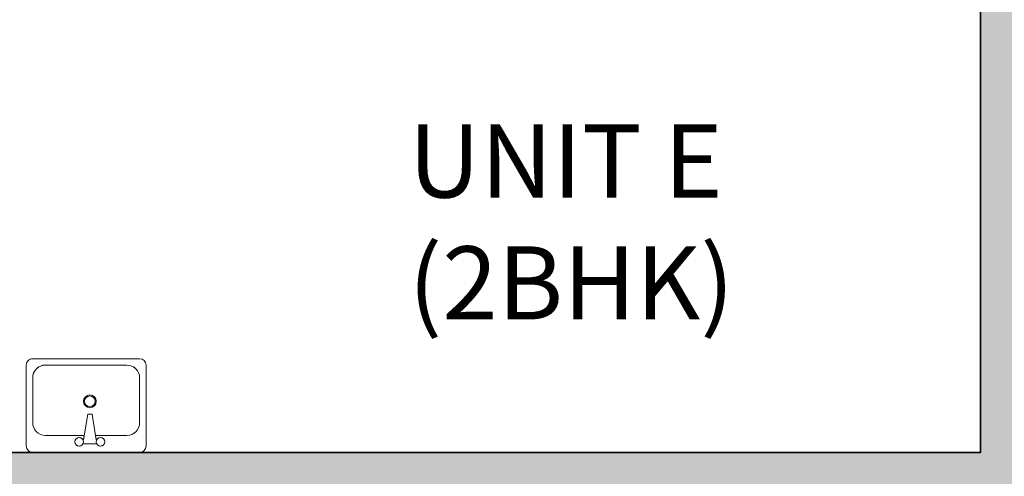
# Model space of a CAD drawing. Units: inches. Extents: x 2083 to 3317, y 1141 to 2115.
# Tile 102 of 256: x 2415 to 2600, y 1707 to 1794. Entities that reach past the tile are written whole.
import ezdxf

# ---------------------------------------------------------------- set-up
doc = ezdxf.new("R2010")
doc.units = ezdxf.units.IN
for name, color, linetype, lineweight in [('A-AREA-IDEN', 7, 'Continuous', 25), ('A-FLOR-FIXT', 9, 'Continuous', 18), ('A-WALL', 7, 'Continuous', 35)]:
    doc.layers.add(name, color=color, linetype=linetype, lineweight=lineweight)
doc.layers.add('A-WALL-PATT', color=251, linetype='Continuous', lineweight=13, true_color=0x636466)
doc.styles.add('DIM_FONT', font='TXT.shx', dxfattribs={"width": 0.8})
doc.styles.get("Standard").update_dxf_attribs({"font": 'arial.ttf'})

# ---------------------------------------------------------------- blocks, each defined once
blk = doc.blocks.new('A$C564A496C')
at = {"linetype": 'ByBlock'}
for p, q in [((543.2, 450), (30.7, 450)), ((0, 419.3), (0, 30.7)), ((238.5, 409.1), (299.8, 409.1)), ((238.5, 388.6), (258.9, 265.9)), ((279.4, 265.9), (299.8, 388.6)), ((573.8, 30.7), (573.8, 419.3)), ((92, 368.2), (243.6, 368.2)), ((294.7, 368.2), (481.8, 368.2)), ((30.7, 92), (30.7, 306.8)), ((543.2, 306.8), (543.2, 92)), ((258.9, 265.9), (279.4, 265.9)), ((30.7, 0), (543.2, 0)), ((481.8, 30.7), (92, 30.7))]:
    blk.add_line(p, q, dxfattribs=at)
for centre, radius in [((218, 398.9), 20.5), ((320.3, 398.9), 20.5), ((269.1, 204.5), 30.7), ((269.1, 204.5), 25.7)]:
    blk.add_circle(centre, radius, dxfattribs=at)
for centre, radius, start, end in [((30.7, 419.3), 30.7, 90, 180), ((543.2, 419.3), 30.7, 0, 90), ((92, 306.8), 61.4, 90, 180), ((481.8, 306.8), 61.4, 0, 90), ((92, 92), 61.4, 180, 270), ((481.8, 92), 61.4, 270, 0), ((30.7, 30.7), 30.7, 180, 270), ((543.2, 30.7), 30.7, 270, 0)]:
    blk.add_arc(centre, radius, start, end, dxfattribs=at)
at = {"style": 'DIM_FONT', "width": 0.8, "flags": 9}
for tag in ['YSIZE', 'XSIZE']:
    blk.add_attdef(tag, (269.1, 450), '', height=0.5, rotation=270, dxfattribs=at)

msp = doc.modelspace()

# ---------------------------------------------------------------- hatches: boundary and pattern name
at = {"layer": 'A-WALL-PATT'}
h = msp.add_hatch(color=256, dxfattribs=at)
h.dxf.hatch_style = 1
h.paths.add_polyline_path([(3126.96, 2020.761), (2748.96, 2020.761), (2604.96, 2020.761), (2226.96, 2020.761), (2226.96, 1702.761), (2466.96, 1702.761), (2466.96, 1582.761), (2418.96, 1582.761), (2418.96, 1477.761), (2226.96, 1477.761), (2226.96, 1263.261), (2544.96, 1263.261), (2544.96, 1411.761), (2604.96, 1411.761), (2685.96, 1411.761), (2685.96, 1420.761), (2604.96, 1420.761), (2604.96, 1573.761), (2604.96, 1702.761), (2604.96, 2011.761), (2748.96, 2011.761), (2748.96, 1702.761), (2862.96, 1702.761), (2862.96, 1621.761), (2871.96, 1621.761), (2871.96, 1702.761), (2883.96, 1702.761), (2883.96, 1706.939, -0.0264593), (2883.96, 1711.761), (2757.96, 1711.761), (2757.96, 1807.761), (2787.96, 1807.761), (2787.96, 1812.261), (2757.96, 1812.261), (2757.96, 2011.761), (2877.96, 2011.761), (2877.96, 1812.261), (2847.96, 1812.261), (2847.96, 1807.761), (2889.836, 1807.761), (2889.836, 1812.261), (2882.46, 1812.261), (2882.46, 2011.761), (3117.96, 2011.761), (3117.96, 1812.261), (2937.836, 1812.261), (2937.836, 1807.761), (2995.71, 1807.761), (2995.71, 1796.118), (3000.21, 1796.118), (3000.21, 1807.761), (3117.96, 1807.761), (3117.96, 1711.761), (3000.21, 1711.761), (3000.21, 1760.118), (2998.573, 1760.118, -0.020711), (2995.71, 1760.118), (2995.71, 1711.761), (2931.96, 1711.761), (2931.96, 1702.761), (3126.96, 1702.761)])
h.paths.add_polyline_path([(2471.46, 2011.761), (2471.46, 1810.011), (2462.717, 1810.011), (2462.717, 1805.511), (2505.96, 1805.511), (2505.96, 1810.011), (2475.96, 1810.011), (2475.96, 2011.761), (2595.96, 2011.761), (2595.96, 1810.011), (2565.96, 1810.011), (2565.96, 1805.511), (2595.96, 1805.511), (2595.96, 1711.761), (2235.96, 1711.761), (2235.96, 1805.511), (2353.71, 1805.511), (2353.71, 1796.054), (2358.21, 1796.054), (2358.21, 1805.511), (2414.717, 1805.511), (2414.717, 1810.011), (2235.96, 1810.011), (2235.96, 2011.761)], flags=16)
h.paths.add_polyline_path([(2270.205, 1994.61), (2270.205, 1970.61), (2246.205, 1970.61), (2246.205, 1994.61)], flags=0)
edge = h.paths.add_edge_path(flags=0)
edge.add_ellipse((2332.027, 1899.798), major_axis=(-3.043, 3.043), ratio=0.1682525, start_angle=-161.33217, end_angle=-156.30711, ccw=False)
edge.add_ellipse((2333.082, 1898.744), major_axis=(-1.055, 1.055), ratio=0.4535321, start_angle=-123.37102, end_angle=-94.15911)
edge = h.paths.add_edge_path(flags=0)
edge.add_ellipse((2332.027, 1968.876), major_axis=(3.043, 3.043), ratio=0.1682525, start_angle=18.66783, end_angle=23.69289)
edge.add_spline(control_points=[(2332.926, 1970.691), (2332.227, 1970.336), (2330.894, 1969.659), (2328.413, 1970.932), (2327.204, 1967.749), (2324.71, 1969.956), (2322.533, 1967.012), (2320.013, 1971.296), (2317.68, 1968.158), (2316.041, 1967.102), (2315.427, 1966.81)], knot_values=[0, 0, 0, 0, 2.2670587, 4.3245589, 6.6855835, 8.8786411, 11.121502, 14.300359, 17.7552837, 19.732645, 19.732645, 19.732645, 19.732645], degree=3, periodic=0)
edge.add_ellipse((2332.027, 1968.876), major_axis=(3.043, 3.043), ratio=0.1682525, start_angle=18.66783, end_angle=23.69289, ccw=False)
edge.add_ellipse((2333.082, 1969.931), major_axis=(1.055, 1.055), ratio=0.4535321, start_angle=56.62898, end_angle=85.84089, ccw=False)
edge = h.paths.add_edge_path(flags=0)
edge.add_spline(control_points=[(2296.428, 1967.988), (2293.628, 1965.336), (2287.704, 1959.727), (2299.744, 1949.996), (2294.533, 1935.669), (2290.573, 1920.604), (2293.394, 1909.974), (2296.185, 1904.967)], knot_values=[0.0991853, 0.0991853, 0.0991853, 0.0991853, 0.3453009, 0.6198217, 0.9826526, 1.3860932, 1.8105546, 1.8105546, 1.8105546, 1.8105546], degree=3, periodic=0)
edge.add_spline(control_points=[(2296.185, 1904.967), (2297.384, 1902.619), (2298.001, 1901.949), (2298.553, 1901.468)], knot_values=[0.0062457, 0.0062457, 0.0062457, 0.0062457, 0.0554759, 0.0554759, 0.0554759, 0.0554759], degree=3, periodic=0)
edge.add_spline(control_points=[(2298.553, 1901.468), (2297.259, 1900.923), (2295.225, 1900.232), (2293.06, 1900.614), (2292.101, 1900.788), (2292.09, 1900.791)], knot_values=[0.3128349, 0.3128349, 0.3128349, 0.3128349, 0.4017797, 0.4749867, 0.4759027, 0.4759027, 0.4759027, 0.4759027], degree=3, periodic=0)
edge.add_arc((2292.794, 1904.664), 3.937, 215.4209, 259.69818, ccw=False)
edge.add_spline(control_points=[(2289.585, 1902.382), (2289.477, 1902.535), (2289.368, 1902.688), (2289.261, 1902.841)], knot_values=[0.1028719, 0.1028719, 0.1028719, 0.1028719, 0.1168958, 0.1168958, 0.1168958, 0.1168958], degree=3, periodic=0)
edge.add_spline(control_points=[(2289.261, 1902.841), (2288.687, 1902.55), (2287.64, 1902.02), (2285.881, 1901.874), (2283.853, 1901.504), (2281.72, 1899.711), (2278.467, 1899.493), (2276.157, 1901.883), (2272.259, 1899.804), (2267.778, 1901.843), (2262.244, 1900.184), (2257.415, 1901.782), (2254.318, 1900.726), (2253.178, 1900.337)], knot_values=[0, 0, 0, 0, 1.9079767, 3.4771759, 5.261074, 7.9728515, 11.6802485, 13.7179214, 16.9395917, 22.789562, 27.5025027, 33.5952153, 37.1456181, 37.1456181, 37.1456181, 37.1456181], degree=3, periodic=0)
edge.add_line((2253.178, 1900.337), (2250.244, 1902.841))
edge.add_line((2250.244, 1902.841), (2250.244, 1965.833))
edge.add_line((2250.244, 1965.833), (2253.178, 1968.337))
edge.add_spline(control_points=[(2253.178, 1968.337), (2254.318, 1967.948), (2257.415, 1966.892), (2262.244, 1968.49), (2267.778, 1966.831), (2271.527, 1968.537), (2273.876, 1967.828), (2274.207, 1967.728)], knot_values=[0, 0, 0, 0, 0.0901802, 0.2449351, 0.3646438, 0.5132331, 0.5378548, 0.5378548, 0.5378548, 0.5378548], degree=3, periodic=0)
edge.add_arc((2274.353, 1963.793), 3.937, 72.05113, 92.12795, ccw=False)
edge.add_arc((2281.297, 1985.23), 18.596, 252.05113, 288.56572)
edge.add_arc((2292.317, 1956.029), 12.646, 71.02679, 113.77822, ccw=False)
edge = h.paths.add_edge_path(flags=0)
edge.add_spline(control_points=[(2274.899, 1951.856), (2275.066, 1951.617), (2275.233, 1951.377), (2275.398, 1951.136)], knot_values=[1.4099157, 1.4099157, 1.4099157, 1.4099157, 1.4315903, 1.4315903, 1.4315903, 1.4315903], degree=3, periodic=0)
edge.add_spline(control_points=[(2275.398, 1951.136), (2275.792, 1950.562), (2276.179, 1949.984), (2276.546, 1949.397)], knot_values=[1.3582378, 1.3582378, 1.3582378, 1.3582378, 1.4099157, 1.4099157, 1.4099157, 1.4099157], degree=3, periodic=0)
edge.add_line((2276.546, 1949.397), (2277.437, 1947.862))
edge.add_spline(control_points=[(2277.437, 1947.862), (2276.304, 1945.673), (2274.64, 1942.427), (2274.632, 1938.094), (2272.799, 1930.852), (2274.356, 1943.897), (2275.948, 1947.923), (2276.546, 1949.397)], knot_values=[0.0056315, 0.0056315, 0.0056315, 0.0056315, 0.1860139, 0.2660015, 0.3570872, 0.5963902, 0.7397317, 0.7397317, 0.7397317, 0.7397317], degree=3, periodic=0)
edge.add_spline(control_points=[(2276.546, 1949.397), (2276.179, 1949.984), (2275.792, 1950.562), (2275.398, 1951.136)], knot_values=[1.3582378, 1.3582378, 1.3582378, 1.3582378, 1.4099157, 1.4099157, 1.4099157, 1.4099157], degree=3, periodic=0)
edge.add_spline(control_points=[(2275.398, 1951.136), (2274.943, 1950.08), (2274.208, 1948.025), (2273.935, 1944.851), (2272.469, 1937.627), (2273.466, 1945.696), (2274.701, 1951.059), (2274.899, 1951.856)], knot_values=[0.1043639, 0.1043639, 0.1043639, 0.1043639, 0.1896363, 0.2696239, 0.3607096, 0.6000126, 0.6446217, 0.6446217, 0.6446217, 0.6446217], degree=3, periodic=0)
h.paths.add_polyline_path([(2269.168, 1963.128, -0.3575267), (2268.171, 1960.976, -0.0925607), (2268.171, 1939.436, -0.3575267), (2269.168, 1937.285, -0.3575267), (2267.016, 1938.282, -0.1647847), (2254.686, 1938.282, -0.3575267), (2252.534, 1937.285, -0.3575267), (2253.531, 1939.436, -0.0925607), (2253.531, 1960.976, -0.3575267), (2252.534, 1963.128, -0.3575267), (2254.686, 1962.131, -0.1647847), (2267.016, 1962.131, -0.3575267)], flags=0)
h.paths.add_polyline_path([(2248.874, 1967.802), (2248.874, 1957.028), (2249.458, 1957.028), (2249.458, 1911.647), (2248.874, 1911.647), (2248.874, 1900.873), (2246.512, 1900.873, 0.1973271), (2244.15, 1902.457), (2244.15, 1966.218, 0.1973271), (2246.512, 1967.802)], flags=0)
h.paths.add_polyline_path([(2269.168, 1931.389, -0.3575267), (2268.171, 1929.238, -0.0925607), (2268.171, 1907.698, -0.3575267), (2269.168, 1905.547, -0.3575267), (2267.016, 1906.544, -0.1647847), (2254.686, 1906.544, -0.3575267), (2252.534, 1905.547, -0.3575267), (2253.531, 1907.698, -0.0925607), (2253.531, 1929.238, -0.3575267), (2252.534, 1931.389, -0.3575267), (2254.686, 1930.392, -0.1647847), (2267.016, 1930.392, -0.3575267)], flags=0)
edge = h.paths.add_edge_path(flags=0)
edge.add_spline(control_points=[(2276.197, 1906.724), (2276.168, 1909.029), (2276.114, 1913.372), (2270.598, 1924.925), (2273.905, 1919.013), (2275.922, 1916.262), (2275.475, 1912.402), (2277.258, 1910.381), (2276.696, 1908.225), (2276.646, 1906.813), (2276.618, 1906.008)], knot_values=[0, 0, 0, 0, 8.6102597, 16.2212739, 18.8430575, 23.8048978, 27.4408283, 29.3561016, 31.2034776, 33.6506866, 33.6506866, 33.6506866, 33.6506866], degree=3, periodic=0)
edge.add_spline(control_points=[(2276.618, 1906.008), (2276.623, 1905.624), (2276.498, 1904.629), (2275.442, 1903.855), (2274.937, 1903.08), (2274.859, 1902.841)], knot_values=[0.1564884, 0.1564884, 0.1564884, 0.1564884, 0.1843975, 0.2313765, 0.2505985, 0.2505985, 0.2505985, 0.2505985], degree=3, periodic=0)
edge.add_line((2274.859, 1902.841), (2276.506, 1902.841))
edge.add_spline(control_points=[(2276.506, 1902.841), (2276.788, 1903.085), (2277.665, 1904.125), (2278.25, 1904.341), (2277.654, 1908.527), (2278.156, 1906.228), (2278.1, 1905.286), (2278.847, 1904.069), (2277.857, 1903.415), (2277.874, 1902.991), (2277.904, 1902.841)], knot_values=[0.0595743, 0.0595743, 0.0595743, 0.0595743, 0.0807529, 0.1037415, 0.1697201, 0.1760361, 0.2071372, 0.2404744, 0.2623409, 0.2736605, 0.2736605, 0.2736605, 0.2736605], degree=3, periodic=0)
edge.add_line((2277.904, 1902.841), (2280.03, 1902.841))
edge.add_spline(control_points=[(2280.03, 1902.841), (2279.888, 1903.088), (2279.499, 1903.982), (2280.152, 1905.939), (2278.104, 1909.658), (2279.762, 1907.185), (2280.328, 1904.875), (2280.485, 1903.49), (2281.463, 1903.249), (2281.758, 1902.936), (2281.834, 1902.841)], knot_values=[0.013856, 0.013856, 0.013856, 0.013856, 0.0348738, 0.0888667, 0.1078792, 0.1267378, 0.158714, 0.1937575, 0.2174868, 0.2267221, 0.2267221, 0.2267221, 0.2267221], degree=3, periodic=0)
edge.add_spline(control_points=[(2281.834, 1902.841), (2281.788, 1902.827), (2281.647, 1902.783), (2281.396, 1902.859), (2281.088, 1902.985), (2280.721, 1903.061), (2280.333, 1903.026), (2280.125, 1902.899), (2280.03, 1902.841)], knot_values=[0, 0, 0, 0, 0.1441304, 0.435517, 0.7492759, 1.1530457, 1.5483707, 1.878348, 1.878348, 1.878348, 1.878348], degree=3, periodic=0)
edge.add_line((2280.03, 1902.841), (2277.904, 1902.841))
edge.add_spline(control_points=[(2277.904, 1902.841), (2277.893, 1902.796), (2277.865, 1902.68), (2277.607, 1902.687), (2277.274, 1902.801), (2276.838, 1902.62), (2276.584, 1902.789), (2276.506, 1902.841)], knot_values=[0, 0, 0, 0, 0.1271885, 0.3261988, 0.6280094, 1.2435704, 1.5153306, 1.5153306, 1.5153306, 1.5153306], degree=3, periodic=0)
edge.add_line((2276.506, 1902.841), (2274.859, 1902.841))
edge.add_spline(control_points=[(2274.859, 1902.841), (2274.814, 1902.899), (2274.725, 1903.013), (2274.493, 1903.119), (2274.244, 1902.961), (2273.937, 1903.185), (2273.614, 1902.983), (2273.408, 1902.883), (2273.322, 1902.841)], knot_values=[0, 0, 0, 0, 0.2184302, 0.4369566, 0.6879766, 0.9903786, 1.3983955, 1.6918498, 1.6918498, 1.6918498, 1.6918498], degree=3, periodic=0)
edge.add_spline(control_points=[(2273.322, 1902.841), (2273.617, 1903.446), (2274.274, 1904.538), (2276.027, 1904.574), (2276.207, 1906.584), (2276.197, 1906.724)], knot_values=[0.0122268, 0.0122268, 0.0122268, 0.0122268, 0.0594721, 0.1062177, 0.134458, 0.134458, 0.134458, 0.134458], degree=3, periodic=0)
h.paths.add_polyline_path([(2270.776, 1897.79), (2270.776, 1873.79), (2246.776, 1873.79), (2246.776, 1897.79)], flags=0)
h.paths.add_polyline_path([(2353.71, 1760.005), (2353.71, 1760.054), (2358.21, 1760.054, -0.033729)], flags=0)
h.paths.add_polyline_path([(2321.819, 1737.529), (2341.995, 1737.529, -0.4142136), (2343.203, 1736.321), (2343.203, 1721.021, -0.4142136), (2341.995, 1719.813), (2321.819, 1719.813, -0.4142136), (2320.611, 1721.021), (2320.611, 1736.321, -0.4142136)], flags=0)
h.paths.add_polyline_path([(2324.235, 1736.321), (2339.579, 1736.321, -0.4142136), (2341.995, 1733.905), (2341.995, 1725.45, -0.4142136), (2339.579, 1723.034), (2333.681, 1723.034), (2333.845, 1722.045, -0.8706461), (2335.425, 1721.826, -0.767327), (2333.923, 1721.423), (2331.291, 1721.423, -0.767327), (2329.788, 1721.826, -0.8706461), (2331.368, 1722.045), (2331.533, 1723.034), (2324.235, 1723.034, -0.4142136), (2321.819, 1725.45), (2321.819, 1733.905, -0.4142136)], flags=0)
h.paths.add_polyline_path([(2570.484, 1928.615), (2589.684, 1928.615), (2590.169, 1928.615), (2590.169, 1904.993), (2570.484, 1904.993)], flags=0)
h.paths.add_polyline_path([(2574.447, 1927.264, -1), (2572.829, 1927.264, -1)], flags=0)
h.paths.add_polyline_path([(2573.09, 1926.941), (2573.925, 1927.776), (2574.148, 1927.553), (2573.313, 1926.718)], flags=0)
h.paths.add_polyline_path([(2578.779, 1919.73, -1), (2571.592, 1919.73, -1)], flags=0)
h.paths.add_polyline_path([(2578.385, 1919.73, -1), (2571.985, 1919.73, -1)], flags=0)
h.paths.add_polyline_path([(2331.596, 1729.476, -1), (2333.618, 1729.476, -1)], flags=0)
h.paths.add_polyline_path([(2578.034, 1927.264, -1), (2576.416, 1927.264, -1)], flags=0)
h.paths.add_polyline_path([(2576.689, 1927.531), (2576.912, 1927.754), (2577.747, 1926.919), (2577.524, 1926.696)], flags=0)
h.paths.add_polyline_path([(2578.139, 1909.86, -1), (2572.232, 1909.86, -1)], flags=0)
h.paths.add_polyline_path([(2577.745, 1909.86, -1), (2572.625, 1909.86, -1)], flags=0)
h.paths.add_polyline_path([(2583.798, 1927.264, -1), (2582.179, 1927.264, -1)], flags=0)
h.paths.add_polyline_path([(2582.719, 1927.754), (2583.554, 1926.919), (2583.331, 1926.696), (2582.496, 1927.531)], flags=0)
h.paths.add_polyline_path([(2582.496, 1927.531), (2582.719, 1927.754), (2583.554, 1926.919), (2583.331, 1926.696)], flags=0)
h.paths.add_polyline_path([(2587.739, 1920.53, -1), (2581.832, 1920.53, -1)], flags=0)
h.paths.add_polyline_path([(2587.345, 1920.53, -1), (2582.225, 1920.53, -1)], flags=0)
h.paths.add_polyline_path([(2587.385, 1927.264, -1), (2585.766, 1927.264, -1)], flags=0)
h.paths.add_polyline_path([(2586.082, 1926.98), (2586.917, 1927.815), (2587.14, 1927.593), (2586.305, 1926.758)], flags=0)
h.paths.add_polyline_path([(2588.379, 1910.66, -1), (2581.192, 1910.66, -1)], flags=0)
h.paths.add_polyline_path([(2587.985, 1910.66, -1), (2581.585, 1910.66, -1)], flags=0)
h.paths.add_polyline_path([(2417.168, 1729.478), (2437.344, 1729.478, -0.4142136), (2438.552, 1728.27), (2438.552, 1712.969, -0.4142136), (2437.344, 1711.761), (2417.168, 1711.761, -0.4142136), (2415.96, 1712.969), (2415.96, 1728.27, -0.4142136)], flags=0)
h.paths.add_polyline_path([(2419.584, 1728.27), (2434.928, 1728.27, -0.4142136), (2437.344, 1725.854), (2437.344, 1717.398, -0.4142136), (2434.928, 1714.983), (2429.029, 1714.983), (2429.194, 1713.994, -0.8706461), (2430.774, 1713.775, -0.767327), (2429.271, 1713.372), (2426.64, 1713.372, -0.767327), (2425.137, 1713.775, -0.8706461), (2426.717, 1713.994), (2426.882, 1714.983), (2419.584, 1714.983, -0.4142136), (2417.168, 1717.398), (2417.168, 1725.854, -0.4142136)], flags=0)
h.paths.add_polyline_path([(2419.584, 1728.27), (2434.928, 1728.27, -0.4142136), (2437.344, 1725.854), (2437.344, 1717.398, -0.4142136), (2434.928, 1714.983), (2429.029, 1714.983), (2428.358, 1719.009), (2427.553, 1719.009), (2426.882, 1714.983), (2419.584, 1714.983, -0.4142136), (2417.168, 1717.398), (2417.168, 1725.854, -0.4142136)], flags=0)
h.paths.add_polyline_path([(2426.944, 1721.425, -1), (2428.967, 1721.425, -1)], flags=0)
h.paths.add_polyline_path([(2475.96, 1702.761), (2595.96, 1702.761), (2595.96, 1582.761), (2475.96, 1582.761)], flags=16)
h.paths.add_polyline_path([(2427.96, 1573.761), (2595.96, 1573.761), (2595.96, 1468.761), (2595.96, 1420.761), (2384.46, 1420.761), (2384.46, 1468.761), (2427.96, 1468.761)], flags=16)
h.paths.add_polyline_path([(2379.96, 1468.761), (2379.96, 1420.761), (2235.96, 1420.761), (2235.96, 1468.761)], flags=16)
h.paths.add_polyline_path([(2317.816, 1466.696), (2337.992, 1466.696, -0.4142136), (2339.2, 1465.488), (2339.2, 1450.187, -0.4142136), (2337.992, 1448.979), (2317.816, 1448.979, -0.4142136), (2316.608, 1450.187), (2316.608, 1465.488, -0.4142136)], flags=0)
h.paths.add_polyline_path([(2320.232, 1465.488), (2335.576, 1465.488, -0.4142136), (2337.992, 1463.072), (2337.992, 1454.616, -0.4142136), (2335.576, 1452.2), (2329.677, 1452.2), (2329.842, 1451.212, -0.8706461), (2331.422, 1450.992, -0.767327), (2329.92, 1450.59), (2327.288, 1450.59, -0.767327), (2325.785, 1450.992, -0.8706461), (2327.365, 1451.212), (2327.53, 1452.2), (2320.232, 1452.2, -0.4142136), (2317.816, 1454.616), (2317.816, 1463.072, -0.4142136)], flags=0)
h.paths.add_polyline_path([(2320.232, 1465.488), (2335.576, 1465.488, -0.4142136), (2337.992, 1463.072), (2337.992, 1454.616, -0.4142136), (2335.576, 1452.2), (2329.677, 1452.2), (2329.006, 1456.227), (2328.201, 1456.227), (2327.53, 1452.2), (2320.232, 1452.2, -0.4142136), (2317.816, 1454.616), (2317.816, 1463.072, -0.4142136)], flags=0)
h.paths.add_polyline_path([(2327.593, 1458.643, -1), (2329.615, 1458.643, -1)], flags=0)
h.paths.add_polyline_path([(2244.412, 1433.34), (2241.921, 1433.34, -0.4142136), (2240.018, 1435.244), (2240.018, 1440.953, -0.4142105), (2241.921, 1442.856), (2244.412, 1442.856, -1.9764724)], flags=0)
h.paths.add_polyline_path([(2245.357, 1434.398, -0.4142136), (2245.357, 1441.799, -2.1440985)], flags=0)
h.paths.add_polyline_path([(2535.96, 1416.261), (2535.96, 1272.261), (2235.96, 1272.261), (2235.96, 1416.261)], flags=16)
h.paths.add_polyline_path([(2260.12, 1384.293), (2260.12, 1362.039), (2237.865, 1362.039), (2237.865, 1384.293)], flags=0)
edge = h.paths.add_edge_path(flags=0)
edge.add_line((2318.252, 1362.093), (2318.146, 1362.001))
edge.add_ellipse((2317.445, 1360.431), major_axis=(2.822, 2.822), ratio=0.1682525, start_angle=18.66783, end_angle=20.94813, ccw=False)
edge.add_ellipse((2318.423, 1361.409), major_axis=(0.978, 0.978), ratio=0.4535321, start_angle=56.62898, end_angle=70.2262, ccw=False)
edge = h.paths.add_edge_path(flags=0)
edge.add_line((2319.107, 1295.571), (2319.015, 1295.677))
edge.add_ellipse((2317.445, 1296.378), major_axis=(-2.822, 2.822), ratio=0.1682525, start_angle=-161.33217, end_angle=-159.05187, ccw=False)
edge.add_ellipse((2318.423, 1295.4), major_axis=(-0.978, 0.978), ratio=0.4535321, start_angle=-123.37102, end_angle=-109.7738)
edge = h.paths.add_edge_path(flags=0)
edge.add_spline(control_points=[(2284.21, 1301.17), (2284.581, 1300.445), (2284.891, 1299.892), (2285.16, 1299.461)], knot_values=[0.0390658, 0.0390658, 0.0390658, 0.0390658, 0.0554759, 0.0554759, 0.0554759, 0.0554759], degree=3, periodic=0)
edge.add_line((2285.16, 1299.461), (2284.21, 1301.17))
edge = h.paths.add_edge_path(flags=0)
edge.add_line((2280.412, 1297.298), (2283.37, 1297.036))
edge.add_line((2283.37, 1297.036), (2286.406, 1297.926))
edge.add_spline(control_points=[(2286.406, 1297.926), (2285.305, 1297.463), (2284.345, 1297.129), (2283.37, 1297.036)], knot_values=[0.3943688, 0.3943688, 0.3943688, 0.3943688, 0.4759027, 0.4759027, 0.4759027, 0.4759027], degree=3, periodic=0)
edge.add_spline(control_points=[(2283.37, 1297.036), (2283.281, 1297.028), (2282.316, 1296.957), (2281.313, 1297.134), (2280.423, 1297.296), (2280.412, 1297.298)], knot_values=[0.3128349, 0.3128349, 0.3128349, 0.3128349, 0.3202458, 0.3934528, 0.3943688, 0.3943688, 0.3943688, 0.3943688], degree=3, periodic=0)
edge = h.paths.add_edge_path(flags=0)
edge.add_line((2284.436, 1359.607), (2280.446, 1355.328))
edge.add_line((2280.446, 1355.328), (2279.58, 1351.018))
edge.add_line((2279.58, 1351.018), (2282.413, 1346.58))
edge.add_spline(control_points=[(2282.413, 1346.58), (2283.153, 1345.589), (2284.253, 1344.029), (2284.801, 1342.387), (2284.935, 1341.806)], knot_values=[1.2400982, 1.2400982, 1.2400982, 1.2400982, 1.3328922, 1.3827123, 1.3827123, 1.3827123, 1.3827123], degree=3, periodic=0)
edge.add_spline(control_points=[(2284.935, 1341.806), (2285.319, 1340.141), (2285.233, 1338.409), (2284.91, 1336.654)], knot_values=[1.0974841, 1.0974841, 1.0974841, 1.0974841, 1.2400982, 1.2400982, 1.2400982, 1.2400982], degree=3, periodic=0)
edge.add_spline(control_points=[(2284.91, 1336.654), (2284.587, 1334.899), (2284.027, 1333.12), (2283.463, 1331.361)], knot_values=[0.9548699, 0.9548699, 0.9548699, 0.9548699, 1.0974841, 1.0974841, 1.0974841, 1.0974841], degree=3, periodic=0)
edge.add_line((2283.463, 1331.361), (2281.89, 1326.153))
edge.add_line((2281.89, 1326.153), (2280.756, 1321.056))
edge.add_line((2280.756, 1321.056), (2280.299, 1316.002))
edge.add_line((2280.299, 1316.002), (2280.716, 1310.95))
edge.add_line((2280.716, 1310.95), (2282.028, 1305.972))
edge.add_line((2282.028, 1305.972), (2284.21, 1301.17))
edge.add_spline(control_points=[(2284.21, 1301.17), (2283.341, 1302.73), (2282.612, 1304.336), (2282.028, 1305.972)], knot_values=[0.0991853, 0.0991853, 0.0991853, 0.0991853, 0.2417994, 0.2417994, 0.2417994, 0.2417994], degree=3, periodic=0)
edge.add_spline(control_points=[(2282.028, 1305.972), (2281.444, 1307.608), (2281.005, 1309.273), (2280.716, 1310.95)], knot_values=[0.2417994, 0.2417994, 0.2417994, 0.2417994, 0.3844135, 0.3844135, 0.3844135, 0.3844135], degree=3, periodic=0)
edge.add_spline(control_points=[(2280.716, 1310.95), (2280.433, 1312.588), (2280.289, 1314.277), (2280.299, 1315.962), (2280.299, 1316.002)], knot_values=[0.3844135, 0.3844135, 0.3844135, 0.3844135, 0.5236467, 0.5270276, 0.5270276, 0.5270276, 0.5270276], degree=3, periodic=0)
edge.add_spline(control_points=[(2280.299, 1316.002), (2280.312, 1317.687), (2280.478, 1319.368), (2280.756, 1321.056)], knot_values=[0.5270276, 0.5270276, 0.5270276, 0.5270276, 0.6696417, 0.6696417, 0.6696417, 0.6696417], degree=3, periodic=0)
edge.add_spline(control_points=[(2280.756, 1321.056), (2281.035, 1322.744), (2281.426, 1324.44), (2281.89, 1326.153)], knot_values=[0.6696417, 0.6696417, 0.6696417, 0.6696417, 0.8122558, 0.8122558, 0.8122558, 0.8122558], degree=3, periodic=0)
edge.add_spline(control_points=[(2281.89, 1326.153), (2282.264, 1327.533), (2282.788, 1329.262), (2283.353, 1331.018), (2283.463, 1331.361)], knot_values=[0.8122558, 0.8122558, 0.8122558, 0.8122558, 0.9270873, 0.9548699, 0.9548699, 0.9548699, 0.9548699], degree=3, periodic=0)
edge.add_line((2283.463, 1331.361), (2284.91, 1336.654))
edge.add_line((2284.91, 1336.654), (2284.935, 1341.806))
edge.add_line((2284.935, 1341.806), (2282.413, 1346.58))
edge.add_spline(control_points=[(2282.413, 1346.58), (2281.275, 1348.104), (2280.078, 1349.57), (2279.58, 1351.018)], knot_values=[1.3827123, 1.3827123, 1.3827123, 1.3827123, 1.5253264, 1.5253264, 1.5253264, 1.5253264], degree=3, periodic=0)
edge.add_spline(control_points=[(2279.58, 1351.018), (2279.443, 1351.415), (2279.136, 1352.857), (2279.735, 1354.29), (2280.446, 1355.328)], knot_values=[1.5253264, 1.5253264, 1.5253264, 1.5253264, 1.564439, 1.6679405, 1.6679405, 1.6679405, 1.6679405], degree=3, periodic=0)
edge.add_spline(control_points=[(2280.446, 1355.328), (2281.426, 1356.758), (2282.931, 1358.183), (2284.436, 1359.607)], knot_values=[1.6679405, 1.6679405, 1.6679405, 1.6679405, 1.8105546, 1.8105546, 1.8105546, 1.8105546], degree=3, periodic=0)
edge.add_arc((2280.623, 1348.518), 11.726, 71.02679, 113.77822)
edge.add_arc((2270.405, 1375.595), 17.244, 252.05113, 288.56572, ccw=False)
edge.add_arc((2263.966, 1355.718), 3.651, 72.05113, 92.12795)
edge.add_arc((2263.966, 1355.718), 3.651, 92.12795, 177.98513)
edge.add_spline(control_points=[(2260.318, 1355.846), (2260.26, 1354.221), (2260.551, 1350.187), (2262.999, 1346.766), (2264.473, 1344.649)], knot_values=[1.4315903, 1.4315903, 1.4315903, 1.4315903, 1.5641438, 1.7706953, 1.7706953, 1.7706953, 1.7706953], degree=3, periodic=0)
edge.add_line((2264.473, 1344.649), (2264.936, 1343.983))
edge.add_spline(control_points=[(2263.801, 1340.248), (2263.843, 1340.514), (2264.067, 1341.756), (2264.513, 1343.002), (2264.935, 1343.981)], knot_values=[0.5365702, 0.5365702, 0.5365702, 0.5365702, 0.5593494, 0.6446217, 0.6446217, 0.6446217, 0.6446217], degree=3, periodic=0)
edge.add_spline(control_points=[(2264.935, 1343.981), (2265.118, 1343.715), (2265.299, 1343.448), (2265.477, 1343.179)], knot_values=[1.3840767, 1.3840767, 1.3840767, 1.3840767, 1.4099157, 1.4099157, 1.4099157, 1.4099157], degree=3, periodic=0)
edge.add_spline(control_points=[(2265.477, 1343.179), (2265.655, 1342.911), (2265.829, 1342.641), (2265.999, 1342.369)], knot_values=[1.3582378, 1.3582378, 1.3582378, 1.3582378, 1.3840767, 1.3840767, 1.3840767, 1.3840767], degree=3, periodic=0)
edge.add_line((2265.999, 1342.369), (2266.826, 1340.946))
edge.add_spline(control_points=[(2266.826, 1340.946), (2268.894, 1337.09), (2271.398, 1325.843), (2270.516, 1310.569), (2275.919, 1301.861), (2277.79, 1299.199)], knot_values=[0.1168958, 0.1168958, 0.1168958, 0.1168958, 0.4729873, 1.0509689, 1.3137934, 1.3137934, 1.3137934, 1.3137934], degree=3, periodic=0)
edge.add_spline(control_points=[(2277.79, 1299.199), (2277.839, 1299.128), (2277.889, 1299.057), (2277.94, 1298.987)], knot_values=[0.1098839, 0.1098839, 0.1098839, 0.1098839, 0.1168958, 0.1168958, 0.1168958, 0.1168958], degree=3, periodic=0)
edge.add_line((2277.94, 1298.987), (2277.789, 1299.199))
edge.add_spline(control_points=[(2277.789, 1299.199), (2277.257, 1298.929), (2276.286, 1298.438), (2275.039, 1298.334), (2274.383, 1298.239), (2274.215, 1298.209)], knot_values=[33.1218702, 33.1218702, 33.1218702, 33.1218702, 35.0290557, 36.5982549, 37.1448269, 37.1448269, 37.1448269, 37.1448269], degree=3, periodic=0)
edge.add_line((2274.215, 1298.209), (2273.073, 1297.893))
edge.add_spline(control_points=[(2273.073, 1297.893), (2272.323, 1297.58), (2271.039, 1296.511), (2269.248, 1296.226), (2268.423, 1296.375)], knot_values=[26.5325843, 26.5325843, 26.5325843, 26.5325843, 29.198919, 31.8391012, 31.8391012, 31.8391012, 31.8391012], degree=3, periodic=0)
edge.add_line((2268.423, 1296.375), (2263.879, 1297.458))
edge.add_spline(control_points=[(2263.879, 1297.458), (2263.556, 1297.359), (2261.86, 1296.839), (2260.239, 1297.282), (2258.933, 1297.516)], knot_values=[15.9195506, 15.9195506, 15.9195506, 15.9195506, 16.9395917, 21.2260675, 21.2260675, 21.2260675, 21.2260675], degree=3, periodic=0)
edge.add_line((2258.933, 1297.516), (2254.055, 1297.329))
edge.add_spline(control_points=[(2254.055, 1297.329), (2253.756, 1297.296), (2252.114, 1297.165), (2250.462, 1297.544), (2249.13, 1297.668)], knot_values=[5.3065169, 5.3065169, 5.3065169, 5.3065169, 6.2764352, 10.6130337, 10.6130337, 10.6130337, 10.6130337], degree=3, periodic=0)
edge.add_line((2249.13, 1297.668), (2244.332, 1296.878))
edge.add_line((2244.332, 1296.878), (2241.611, 1299.199))
edge.add_line((2241.611, 1299.199), (2241.611, 1357.609))
edge.add_line((2241.611, 1357.609), (2244.332, 1359.931))
edge.add_line((2244.332, 1359.931), (2252.729, 1359.543))
edge.add_spline(control_points=[(2252.729, 1359.543), (2252.871, 1359.546), (2253.306, 1359.548), (2253.74, 1359.514), (2254.032, 1359.482)], knot_values=[0.233291, 0.233291, 0.233291, 0.233291, 0.2449351, 0.2689274, 0.2689274, 0.2689274, 0.2689274], degree=3, periodic=0)
edge.add_line((2254.032, 1359.482), (2259.587, 1359.416))
edge.add_spline(control_points=[(2259.587, 1359.416), (2260.677, 1359.629), (2262.073, 1359.897), (2263.524, 1359.459), (2263.83, 1359.366)], knot_values=[0.4225164, 0.4225164, 0.4225164, 0.4225164, 0.5132331, 0.5378548, 0.5378548, 0.5378548, 0.5378548], degree=3, periodic=0)
edge.add_arc((2263.966, 1355.718), 3.651, 72.05113, 92.12795, ccw=False)
edge.add_arc((2270.405, 1375.595), 17.244, 252.05113, 288.56572)
edge.add_arc((2280.623, 1348.518), 11.726, 71.02679, 113.77822, ccw=False)
h.paths.add_polyline_path([(2240.341, 1359.435), (2240.341, 1349.444), (2240.882, 1349.444), (2240.882, 1307.365), (2240.341, 1307.365), (2240.341, 1297.374), (2238.15, 1297.374, 0.1973271), (2235.96, 1298.843), (2235.96, 1357.966, 0.1973271), (2238.15, 1359.435)], flags=0)
h.paths.add_polyline_path([(2259.158, 1355.101, -0.3575267), (2258.233, 1353.106, -0.0925607), (2258.233, 1333.133, -0.3575267), (2259.158, 1331.138, -0.3575267), (2257.163, 1332.062, -0.1647847), (2245.729, 1332.062, -0.3575267), (2243.735, 1331.138, -0.3575267), (2244.659, 1333.133, -0.0925607), (2244.659, 1353.106, -0.3575267), (2243.735, 1355.101, -0.3575267), (2245.729, 1354.176, -0.1647847), (2257.163, 1354.176, -0.3575267)], flags=0)
edge = h.paths.add_edge_path(flags=0)
edge.add_line((2265.999, 1342.369), (2266.826, 1340.946))
edge.add_line((2266.826, 1340.946), (2265.308, 1337.814))
edge.add_line((2265.308, 1337.814), (2264.358, 1334.653))
edge.add_line((2264.358, 1334.653), (2264.262, 1333.8))
edge.add_spline(control_points=[(2264.262, 1333.8), (2264.208, 1333.187), (2264.162, 1332.366), (2264.007, 1331.414), (2263.969, 1331.202)], knot_values=[0.4644442, 0.4644442, 0.4644442, 0.4644442, 0.5166905, 0.5316081, 0.5316081, 0.5316081, 0.5316081], degree=3, periodic=0)
edge.add_spline(control_points=[(2263.969, 1331.202), (2263.775, 1330.119), (2263.424, 1328.791), (2263.257, 1328.531), (2263.234, 1328.515)], knot_values=[0.3726816, 0.3726816, 0.3726816, 0.3726816, 0.4488497, 0.4644442, 0.4644442, 0.4644442, 0.4644442], degree=3, periodic=0)
edge.add_spline(control_points=[(2263.234, 1328.515), (2263.096, 1328.42), (2263.131, 1329.301), (2263.275, 1330.616)], knot_values=[0.2809191, 0.2809191, 0.2809191, 0.2809191, 0.3726816, 0.3726816, 0.3726816, 0.3726816], degree=3, periodic=0)
edge.add_spline(control_points=[(2263.275, 1330.616), (2263.419, 1331.93), (2263.672, 1333.677), (2263.97, 1335.315)], knot_values=[0.1891566, 0.1891566, 0.1891566, 0.1891566, 0.2809191, 0.2809191, 0.2809191, 0.2809191], degree=3, periodic=0)
edge.add_spline(control_points=[(2263.97, 1335.315), (2264.1, 1336.032), (2264.419, 1337.622), (2264.755, 1338.864), (2264.947, 1339.491)], knot_values=[0.097394, 0.097394, 0.097394, 0.097394, 0.1375775, 0.1891566, 0.1891566, 0.1891566, 0.1891566], degree=3, periodic=0)
edge.add_spline(control_points=[(2264.947, 1339.491), (2265.29, 1340.606), (2265.644, 1341.494), (2265.999, 1342.369)], knot_values=[0.0056315, 0.0056315, 0.0056315, 0.0056315, 0.097394, 0.097394, 0.097394, 0.097394], degree=3, periodic=0)
h.paths.add_polyline_path([(2259.158, 1325.671, -0.3575267), (2258.233, 1323.676, -0.0925607), (2258.233, 1303.703, -0.3575267), (2259.158, 1301.708, -0.3575267), (2257.163, 1302.633, -0.1647847), (2245.729, 1302.633, -0.3575267), (2243.735, 1301.708, -0.3575267), (2244.659, 1303.703, -0.0925607), (2244.659, 1323.676, -0.3575267), (2243.735, 1325.671, -0.3575267), (2245.729, 1324.747, -0.1647847), (2257.163, 1324.747, -0.3575267)], flags=0)
edge = h.paths.add_edge_path(flags=0)
edge.add_spline(control_points=[(2261.709, 1317.311), (2261.679, 1317.418), (2261.762, 1317.389), (2262.491, 1316.09), (2262.962, 1315.301)], knot_values=[14.9558607, 14.9558607, 14.9558607, 14.9558607, 16.2212739, 18.6948259, 18.6948259, 18.6948259, 18.6948259], degree=3, periodic=0)
edge.add_spline(control_points=[(2262.962, 1315.301), (2262.99, 1315.254), (2263.702, 1314.067), (2264.349, 1313.127), (2264.73, 1312.164)], knot_values=[18.6948259, 18.6948259, 18.6948259, 18.6948259, 18.8430575, 22.433791, 22.433791, 22.433791, 22.433791], degree=3, periodic=0)
edge.add_spline(control_points=[(2264.73, 1312.164), (2264.876, 1311.796), (2265.177, 1310.77), (2265.143, 1309.559), (2265.248, 1308.824)], knot_values=[22.433791, 22.433791, 22.433791, 22.433791, 23.8048978, 26.1727562, 26.1727562, 26.1727562, 26.1727562], degree=3, periodic=0)
edge.add_line((2265.248, 1308.824), (2265.851, 1307.172))
edge.add_spline(control_points=[(2265.851, 1307.172), (2266.065, 1306.822), (2266.384, 1306.332), (2266.424, 1305.781), (2266.42, 1305.611)], knot_values=[28.0625624, 28.0625624, 28.0625624, 28.0625624, 29.3561016, 29.9117214, 29.9117214, 29.9117214, 29.9117214], degree=3, periodic=0)
edge.add_spline(control_points=[(2266.42, 1305.611), (2266.416, 1305.433), (2266.394, 1305.25), (2266.365, 1305.066)], knot_values=[29.9117214, 29.9117214, 29.9117214, 29.9117214, 30.4978371, 30.4978371, 30.4978371, 30.4978371], degree=3, periodic=0)
edge.add_line((2266.365, 1305.066), (2266.066, 1302.136))
edge.add_spline(control_points=[(2266.066, 1302.136), (2266.071, 1301.78), (2265.998, 1301.2), (2265.663, 1300.759), (2265.509, 1300.586)], knot_values=[0.1564884, 0.1564884, 0.1564884, 0.1564884, 0.1843975, 0.2035434, 0.2035434, 0.2035434, 0.2035434], degree=3, periodic=0)
edge.add_line((2265.509, 1300.586), (2264.435, 1299.199))
edge.add_line((2264.435, 1299.199), (2265.962, 1299.199))
edge.add_line((2265.962, 1299.199), (2267.336, 1301.175))
edge.add_line((2267.336, 1301.175), (2267.312, 1301.986))
edge.add_spline(control_points=[(2267.312, 1301.986), (2267.261, 1302.862), (2267.16, 1303.737), (2267.271, 1303.326)], knot_values=[0.1262286, 0.1262286, 0.1262286, 0.1262286, 0.1666174, 0.1666174, 0.1666174, 0.1666174], degree=3, periodic=0)
edge.add_spline(control_points=[(2267.271, 1303.326), (2267.28, 1303.294), (2267.31, 1303.175), (2267.373, 1302.884), (2267.406, 1302.683), (2267.418, 1302.601)], knot_values=[0.1666174, 0.1666174, 0.1666174, 0.1666174, 0.1697201, 0.1760361, 0.1807647, 0.1807647, 0.1807647, 0.1807647], degree=3, periodic=0)
edge.add_spline(control_points=[(2267.744, 1300.988), (2267.688, 1301.151), (2267.481, 1301.657), (2267.484, 1302.145), (2267.418, 1302.601)], knot_values=[0.1807647, 0.1807647, 0.1807647, 0.1807647, 0.1937665, 0.2201389, 0.2201389, 0.2201389, 0.2201389], degree=3, periodic=0)
edge.add_line((2267.418, 1302.601), (2267.744, 1300.988))
edge.add_spline(control_points=[(2267.744, 1300.988), (2267.832, 1300.732), (2267.932, 1300.31), (2267.555, 1299.975), (2267.429, 1299.829)], knot_values=[0.2201389, 0.2201389, 0.2201389, 0.2201389, 0.2404744, 0.2548903, 0.2548903, 0.2548903, 0.2548903], degree=3, periodic=0)
edge.add_line((2267.429, 1299.829), (2267.258, 1299.199))
edge.add_line((2267.258, 1299.199), (2269.23, 1299.199))
edge.add_spline(control_points=[(2269.23, 1299.199), (2269.099, 1299.429), (2268.843, 1300.016), (2269.012, 1300.916), (2268.947, 1301.661)], knot_values=[0.013856, 0.013856, 0.013856, 0.013856, 0.0348738, 0.0670726, 0.0670726, 0.0670726, 0.0670726], degree=3, periodic=0)
edge.add_line((2268.947, 1301.661), (2268.432, 1303.603))
edge.add_spline(control_points=[(2268.432, 1303.603), (2268.176, 1304.192), (2267.596, 1305.251), (2268.041, 1304.623), (2268.251, 1304.282)], knot_values=[0.0901547, 0.0901547, 0.0901547, 0.0901547, 0.1078792, 0.1202891, 0.1202891, 0.1202891, 0.1202891], degree=3, periodic=0)
edge.add_spline(control_points=[(2268.251, 1304.282), (2268.361, 1304.105), (2269.058, 1302.918), (2269.383, 1301.59), (2269.521, 1300.776), (2269.575, 1300.556)], knot_values=[0.1202891, 0.1202891, 0.1202891, 0.1202891, 0.1267378, 0.158714, 0.1735056, 0.1735056, 0.1735056, 0.1735056], degree=3, periodic=0)
edge.add_line((2269.575, 1300.556), (2270.686, 1299.421))
edge.add_spline(control_points=[(2270.686, 1299.421), (2270.767, 1299.357), (2270.838, 1299.281), (2270.903, 1299.199)], knot_values=[0.2181597, 0.2181597, 0.2181597, 0.2181597, 0.2267221, 0.2267221, 0.2267221, 0.2267221], degree=3, periodic=0)
edge.add_line((2270.937, 1299.193), (2270.903, 1299.199))
edge.add_spline(control_points=[(2270.903, 1299.199), (2270.86, 1299.186), (2270.73, 1299.146), (2270.496, 1299.216), (2270.272, 1299.308), (2270.121, 1299.348), (2270.063, 1299.36)], knot_values=[0.939174, 0.939174, 0.939174, 0.939174, 1.0833044, 1.3746911, 1.6884499, 1.878348, 1.878348, 1.878348, 1.878348], degree=3, periodic=0)
edge.add_line((2270.063, 1299.36), (2269.23, 1299.199))
edge.add_line((2269.23, 1299.199), (2267.258, 1299.199))
edge.add_spline(control_points=[(2267.258, 1299.199), (2267.248, 1299.157), (2267.223, 1299.05), (2266.984, 1299.057), (2266.809, 1299.116), (2266.677, 1299.109), (2266.637, 1299.105)], knot_values=[0.7576653, 0.7576653, 0.7576653, 0.7576653, 0.8848538, 1.0838641, 1.3856747, 1.5153306, 1.5153306, 1.5153306, 1.5153306], degree=3, periodic=0)
edge.add_spline(control_points=[(2266.637, 1299.105), (2266.485, 1299.089), (2266.236, 1299.017), (2266.035, 1299.151), (2265.962, 1299.199)], knot_values=[0, 0, 0, 0, 0.4859051, 0.7576653, 0.7576653, 0.7576653, 0.7576653], degree=3, periodic=0)
edge.add_line((2265.962, 1299.199), (2264.435, 1299.199))
edge.add_line((2264.435, 1299.199), (2263.858, 1299.367))
edge.add_spline(control_points=[(2263.858, 1299.367), (2263.819, 1299.371), (2263.78, 1299.386), (2263.74, 1299.402)], knot_values=[0.8459249, 0.8459249, 0.8459249, 0.8459249, 0.9786272, 0.9786272, 0.9786272, 0.9786272], degree=3, periodic=0)
edge.add_line((2263.722, 1299.396), (2263.01, 1299.199))
edge.add_spline(control_points=[(2263.01, 1299.199), (2263.246, 1299.683), (2263.506, 1300.128), (2263.873, 1300.408)], knot_values=[0.0122268, 0.0122268, 0.0122268, 0.0122268, 0.0529705, 0.0529705, 0.0529705, 0.0529705], degree=3, periodic=0)
edge.add_spline(control_points=[(2263.873, 1300.408), (2263.932, 1300.453), (2264.084, 1300.553), (2264.255, 1300.624), (2264.36, 1300.665)], knot_values=[0.0529705, 0.0529705, 0.0529705, 0.0529705, 0.0594721, 0.0690861, 0.0690861, 0.0690861, 0.0690861], degree=3, periodic=0)
edge.add_line((2264.36, 1300.665), (2265.142, 1301.078))
edge.add_line((2265.142, 1301.078), (2265.676, 1302.8))
edge.add_line((2265.676, 1302.8), (2265.541, 1305.704))
edge.add_line((2265.541, 1305.704), (2264.803, 1309.328))
edge.add_line((2264.803, 1309.328), (2263.041, 1314.092))
edge.add_spline(control_points=[(2263.041, 1314.092), (2262.384, 1315.671), (2261.796, 1316.998), (2261.709, 1317.311)], knot_values=[11.2168955, 11.2168955, 11.2168955, 11.2168955, 14.9558607, 14.9558607, 14.9558607, 14.9558607], degree=3, periodic=0)
h.paths.add_polyline_path([(2871.96, 1416.261), (2895.91, 1416.261), (2895.91, 1420.761), (2871.96, 1420.761), (2871.96, 1501.761), (2862.96, 1501.761), (2862.96, 1420.761), (2805.96, 1420.761), (2805.96, 1411.761), (2862.96, 1411.761), (2862.96, 1263.261), (3126.96, 1263.261), (3126.96, 1411.761), (3126.96, 1486.761), (2943.96, 1486.761), (2943.96, 1477.761), (2967.86, 1477.761), (2967.86, 1420.761), (2943.91, 1420.761), (2943.91, 1416.261), (3117.96, 1416.261), (3117.96, 1420.761), (2972.36, 1420.761), (2972.36, 1477.761), (3117.96, 1477.761), (3117.96, 1420.761), (3117.96, 1272.261), (2871.96, 1272.261)], flags=0)
h.paths.add_polyline_path([(2457.126, 1485.943), (2527.603, 1485.943), (2527.603, 1537.636), (2457.126, 1537.636)], flags=8)
h.paths.add_polyline_path([(2481.005, 1609.982), (2590.766, 1609.982), (2590.766, 1682.003), (2481.005, 1682.003)], flags=8)
h.paths.add_polyline_path([(2483.085, 1729.127), (2553.562, 1729.127), (2553.562, 1780.82), (2483.085, 1780.82)], flags=8)

# ---------------------------------------------------------------- linework, layer by layer
at = {"layer": 'A-FLOR-FIXT'}
for p, q in [((2419.584, 1728.27), (2434.928, 1728.27)), ((2417.168, 1717.398), (2417.168, 1725.854)), ((2437.344, 1725.854), (2437.344, 1717.398)), ((2426.882, 1714.983), (2419.584, 1714.983)), ((2426.717, 1713.994), (2426.882, 1714.983)), ((2434.928, 1714.983), (2429.029, 1714.983)), ((2429.029, 1714.983), (2429.194, 1713.994)), ((2429.271, 1713.372), (2426.64, 1713.372))]:
    msp.add_line(p, q, dxfattribs=at)
for centre, radius, start, end in [((2419.584, 1725.854), 2.416, 90, 180), ((2434.928, 1725.854), 2.416, 0, 90), ((2427.955, 1721.425), 1.011, 0, 180), ((2427.955, 1721.425), 1.011, 180, 0), ((2419.584, 1717.398), 2.416, 180, 270), ((2434.928, 1717.398), 2.416, 270, 360), ((2425.942, 1713.775), 0.805, 15.82267, 180), ((2429.969, 1713.775), 0.805, 0, 164.17733), ((2425.942, 1713.775), 0.805, 180, 330), ((2429.969, 1713.775), 0.805, 210, 0)]:
    msp.add_arc(centre, radius, start, end, dxfattribs=at)
at = {"layer": 'A-WALL'}
for p in [(2595.96, 1805.511), (2235.96, 1711.761)]:
    msp.add_line(p, (2595.96, 1711.761), dxfattribs=at)

# ---------------------------------------------------------------- block references
at = {"layer": 'A-FLOR-FIXT', "xscale": 0.0393700787401575, "yscale": 0.0393700787401575, "zscale": 0.0393700787401575, "rotation": 180}
msp.add_blockref('A$C564A496C', (2438.552, 1729.478), dxfattribs=at)

# ---------------------------------------------------------------- texts
at = {"layer": 'A-AREA-IDEN', "insert": (2488.053, 1773.715), "char_height": 13.8054, "attachment_point": 1}
msp.add_mtext_dynamic_manual_height_columns('UNIT E \\P(2BHK)', width=250.71568, gutter_width=69.027, heights=[0], dxfattribs=at)

doc.saveas('drawing.dxf')
